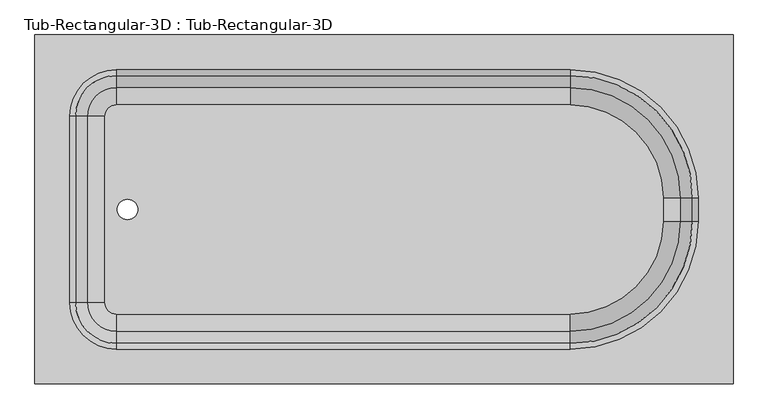
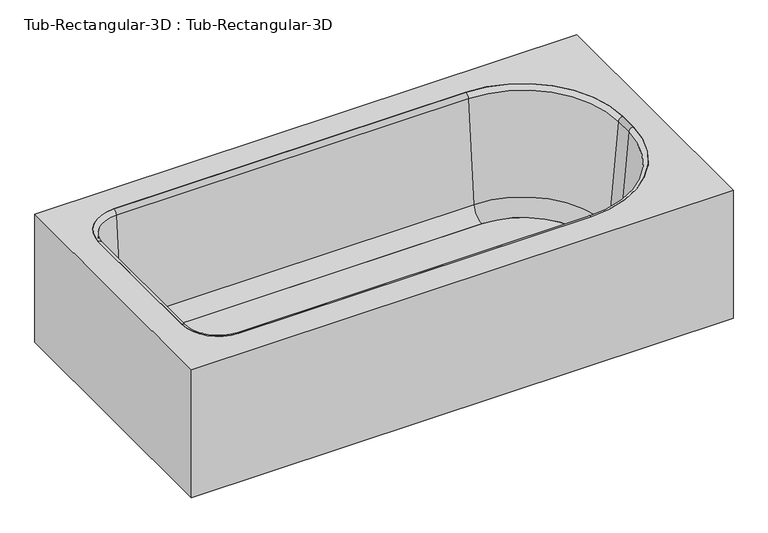
"""IFC4 building model written with IfcOpenShell, lengths in millimetres: flow terminal geometry, Tub-Rectangular-3D : Tub-Rectangular-3D."""

from ifc_helpers import new_model, si_unit, point, frame, frame_2d, origin, place, context, project, spatial, polyline, circle_curve, ellipse_curve, trimmed, segment, composite_curve, outline, extrude, source, transform, mapped, element, save
from ifc_brep_helpers import plane_surface, cylinder_surface, revolved_surface, advanced_brep


def tub_rectangular_3d_tub_rectangular_3d_c1fa07c3(model_context):
    return source(origin(), model_context, "Body", "SolidModel", [
        advanced_brep(
        [(413.3970313, -863.6, 381.0), (413.3970313, -101.6, 381.0), (-1110.6029687, -101.6, 381.0), (-1110.6029687, -863.6, 381.0), (-932.8029687, -787.4, 381.0), (-1034.4029687, -685.8, 381.0), (-1034.4029687, -279.4, 381.0), (-932.8029687, -177.8, 381.0), (57.7970313, -177.8, 381.0), (337.1970313, -457.2, 381.0), (337.1970313, -508.0, 381.0), (57.7970313, -787.4, 381.0), (394.3470313, -844.55, 361.95), (-1091.5529687, -844.55, 361.95), (-1091.5529687, -120.65, 361.95), (394.3470313, -120.65, 361.95), (-932.8029687, -787.4, 361.95), (57.7970313, -787.4, 361.95), (337.1970313, -508.0, 361.95), (337.1970313, -457.2, 361.95), (57.7970313, -177.8, 361.95), (-932.8029687, -177.8, 361.95), (-1034.4029687, -279.4, 361.95), (-1034.4029687, -685.8, 361.95), (-1110.6029687, -863.6, 0.0), (413.3970313, -863.6, 0.0), (-1110.6029687, -101.6, 0.0), (413.3970313, -101.6, 0.0), (394.3470313, -844.55, 0.0), (394.3470313, -120.65, 0.0), (-1091.5529687, -120.65, 0.0), (-1091.5529687, -844.55, 0.0)],
        [
            (0, 1),
            (1, 2),
            (2, 3),
            (3, 0),
            (4, 5, circle_curve(frame((-932.8029687, -685.8, 381.0), z_axis=(0.0, 0.0, -1.0), x_axis=(0.0, -1.0, 0.0)), 101.6)),
            (5, 6),
            (6, 7, circle_curve(frame((-932.8029687, -279.4, 381.0), z_axis=(0.0, 0.0, -1.0), x_axis=(0.0, -1.0, 0.0)), 101.6)),
            (7, 8),
            (8, 9, circle_curve(frame((57.7970313, -457.2, 381.0), z_axis=(0.0, 0.0, -1.0), x_axis=(0.0, -1.0, 0.0)), 279.4)),
            (9, 10),
            (10, 11, circle_curve(frame((57.7970313, -508.0, 381.0), z_axis=(0.0, 0.0, -1.0), x_axis=(0.0, -1.0, 0.0)), 279.4)),
            (11, 4),
            (12, 13),
            (13, 14),
            (14, 15),
            (15, 12),
            (16, 17),
            (17, 18, circle_curve(frame((57.7970313, -508.0, 361.95), z_axis=(0.0, 0.0, 1.0), x_axis=(0.0, -1.0, 0.0)), 279.4)),
            (18, 19),
            (19, 20, circle_curve(frame((57.7970313, -457.2, 361.95), z_axis=(0.0, 0.0, 1.0), x_axis=(0.0, -1.0, 0.0)), 279.4)),
            (20, 21),
            (21, 22, circle_curve(frame((-932.8029687, -279.4, 361.95), z_axis=(0.0, 0.0, 1.0), x_axis=(0.0, -1.0, 0.0)), 101.6)),
            (22, 23),
            (23, 16, circle_curve(frame((-932.8029687, -685.8, 361.95), z_axis=(0.0, 0.0, 1.0), x_axis=(0.0, -1.0, 0.0)), 101.6)),
            (3, 24),
            (24, 25),
            (25, 0),
            (2, 26),
            (26, 24),
            (1, 27),
            (27, 26),
            (25, 27),
            (11, 17),
            (16, 4),
            (10, 18),
            (9, 19),
            (8, 20),
            (7, 21),
            (6, 22),
            (5, 23),
            (28, 29),
            (29, 30),
            (30, 31),
            (31, 28),
            (28, 12),
            (15, 29),
            (14, 30),
            (13, 31),
        ],
        [
            plane_surface(frame((-1110.6029687, -863.6, 381.0), z_axis=(0.0, 0.0, 1.0), x_axis=(-1.0, 0.0, 0.0))),
            plane_surface(frame((-1110.6029687, -863.6, 361.95), z_axis=(0.0, 0.0, -1.0), x_axis=(1.0, 0.0, 0.0))),
            plane_surface(frame((413.3970313, -863.6, 381.0), z_axis=(0.0, -1.0, 0.0), x_axis=(0.0, 0.0, -1.0))),
            plane_surface(frame((-1110.6029687, -863.6, 381.0), z_axis=(-1.0, 0.0, 0.0), x_axis=(0.0, 0.0, -1.0))),
            plane_surface(frame((-1110.6029687, -101.6, 381.0), z_axis=(0.0, 1.0, 0.0), x_axis=(0.0, 0.0, -1.0))),
            plane_surface(frame((413.3970313, -101.6, 381.0), z_axis=(1.0, 0.0, 0.0), x_axis=(0.0, 0.0, -1.0))),
            plane_surface(frame((-932.8029687, -787.4, 381.0), z_axis=(0.0, 1.0, 0.0), x_axis=(0.0, 0.0, -1.0))),
            revolved_surface(polyline([(57.7970313, -787.4, 361.95), (57.7970313, -787.4, 381.0)]), (57.7970313, -508.0, 381.0), (0.0, 0.0, -1.0)),
            plane_surface(frame((337.1970313, -508.0, 381.0), z_axis=(-1.0, 0.0, 0.0), x_axis=(0.0, 0.0, -1.0))),
            revolved_surface(polyline([(57.7970313, -736.5999999999999, 361.95), (57.7970313, -736.5999999999999, 381.0)]), (57.7970313, -457.2, 381.0), (0.0, 0.0, -1.0)),
            plane_surface(frame((57.7970313, -177.8, 381.0), z_axis=(0.0, -1.0, 0.0), x_axis=(0.0, 0.0, -1.0))),
            revolved_surface(polyline([(-932.8029687, -381.0, 361.95), (-932.8029687, -381.0, 381.0)]), (-932.8029687, -279.4, 381.0), (0.0, 0.0, -1.0)),
            plane_surface(frame((-1034.4029687, -279.4, 381.0), z_axis=(1.0, 0.0, 0.0), x_axis=(0.0, 0.0, -1.0))),
            revolved_surface(polyline([(-932.8029687, -787.4, 361.95), (-932.8029687, -787.4, 381.0)]), (-932.8029687, -685.8, 381.0), (0.0, 0.0, -1.0)),
            plane_surface(frame((-1110.6029687, -863.6, 0.0), z_axis=(0.0, 0.0, -1.0), x_axis=(1.0, 0.0, 0.0))),
            plane_surface(frame((394.3470313, -844.55, 361.95), z_axis=(-1.0, 0.0, 0.0), x_axis=(0.0, 0.0, -1.0))),
            plane_surface(frame((394.3470313, -120.65, 361.95), z_axis=(0.0, -1.0, 0.0), x_axis=(0.0, 0.0, -1.0))),
            plane_surface(frame((-1091.5529687, -120.65, 361.95), z_axis=(1.0, 0.0, 0.0), x_axis=(0.0, 0.0, -1.0))),
            plane_surface(frame((-1091.5529687, -844.55, 361.95), z_axis=(0.0, 1.0, 0.0), x_axis=(0.0, 0.0, -1.0))),
        ],
        [
            (0, [[1, 2, 3, 4], [5, 6, 7, 8, 9, 10, 11, 12]]),
            (1, [[13, 14, 15, 16], [17, 18, 19, 20, 21, 22, 23, 24]]),
            (2, [[25, 26, 27, -4]]),
            (3, [[28, 29, -25, -3]]),
            (4, [[30, 31, -28, -2]]),
            (5, [[32, -30, -1, -27]]),
            (6, [[33, -17, 34, -12]]),
            (7, [[35, -18, -33, -11]]),
            (8, [[36, -19, -35, -10]]),
            (9, [[37, -20, -36, -9]]),
            (10, [[38, -21, -37, -8]]),
            (11, [[39, -22, -38, -7]]),
            (12, [[40, -23, -39, -6]]),
            (13, [[-34, -24, -40, -5]]),
            (14, [[-26, -29, -31, -32], [41, 42, 43, 44]]),
            (15, [[45, -16, 46, -41]]),
            (16, [[-46, -15, 47, -42]]),
            (17, [[-47, -14, 48, -43]]),
            (18, [[-48, -13, -45, -44]]),
        ],
    ),
        extrude(outline(composite_curve([segment(polyline([(57.7970313, -710.7964741), (-932.8029687, -710.7964741)]), True, "CONTINUOUS"), segment(trimmed(circle_curve(frame_2d((-932.8029687, -685.8)), 24.9964741), [point((-932.8029687, -710.7964741))], [point((-957.7994428, -685.8))], False, "CARTESIAN"), True, "CONTINUOUS"), segment(polyline([(-957.7994428, -685.8), (-957.7994428, -279.4)]), True, "CONTINUOUS"), segment(trimmed(circle_curve(frame_2d((-932.8029687, -279.4)), 24.9964741), [point((-957.7994428, -279.4))], [point((-932.8029687, -254.4035259))], False, "CARTESIAN"), True, "CONTINUOUS"), segment(polyline([(-932.8029687, -254.4035259), (57.7970313, -254.4035259)]), True, "CONTINUOUS"), segment(trimmed(circle_curve(frame_2d((57.7970313, -457.2)), 202.7964741), [point((57.7970313, -254.4035259))], [point((260.5935054, -457.2))], False, "CARTESIAN"), True, "CONTINUOUS"), segment(polyline([(260.5935054, -457.2), (260.5935054, -508.0)]), True, "CONTINUOUS"), segment(trimmed(circle_curve(frame_2d((57.7970313, -508.0)), 202.7964741), [point((260.5935054, -508.0))], [point((57.7970313, -710.7964741))], False, "CARTESIAN"), True, "CONTINUOUS")], self_intersect=False), holes=[composite_curve([segment(trimmed(circle_curve(frame_2d((-908.510206, -482.6)), 22.225), [point((-908.510206, -504.825))], [point((-908.510206, -460.375))], True, "CARTESIAN"), True, "CONTINUOUS"), segment(trimmed(circle_curve(frame_2d((-908.510206, -482.6)), 22.225), [point((-908.510206, -460.375))], [point((-908.510206, -504.825))], True, "CARTESIAN"), True, "CONTINUOUS")], self_intersect=False)]), frame((0.0, 0.0, 16.863573), z_axis=(0.0, 0.0, 1.0), x_axis=(1.0, 0.0, 0.0)), (0.0, 0.0, 1.0), 19.05),
        advanced_brep(
        [(-995.7544608, -685.8, 70.6929392), (-1021.9249722, -685.8, 369.8232535), (-932.8029687, -774.9220035, 369.8232535), (-932.8029687, -748.7514921, 70.6929392), (-957.7994428, -685.8, 35.913573), (-932.8029687, -710.7964741, 35.913573), (-957.7994428, -685.8, 16.863573), (-932.8029687, -710.7964741, 16.863573), (-1034.4029687, -685.8, 16.863573), (-932.8029687, -787.4, 16.863573), (-1034.4029687, -685.8, 381.0), (-932.8029687, -787.4, 381.0), (-995.7544608, -279.4, 70.6929392), (-1021.9249722, -279.4, 369.8232535), (-957.7994428, -279.4, 35.913573), (-957.7994428, -279.4, 16.863573), (-1034.4029687, -279.4, 16.863573), (-1034.4029687, -279.4, 381.0), (-932.8029687, -216.4485079, 70.6929392), (-932.8029687, -190.2779965, 369.8232535), (-932.8029687, -254.4035259, 35.913573), (-932.8029687, -254.4035259, 16.863573), (-932.8029687, -177.8, 16.863573), (-932.8029687, -177.8, 381.0), (57.7970313, -216.4485079, 70.6929392), (57.7970313, -190.2779965, 369.8232535), (57.7970313, -254.4035259, 35.913573), (57.7970313, -254.4035259, 16.863573), (57.7970313, -177.8, 16.863573), (57.7970313, -177.8, 381.0), (298.5485234, -457.2, 70.6929392), (324.7190348, -457.2, 369.8232535), (260.5935054, -457.2, 35.913573), (260.5935054, -457.2, 16.863573), (337.1970313, -457.2, 16.863573), (337.1970313, -457.2, 381.0), (298.5485234, -508.0, 70.6929392), (324.7190348, -508.0, 369.8232535), (260.5935054, -508.0, 35.913573), (260.5935054, -508.0, 16.863573), (337.1970313, -508.0, 16.863573), (337.1970313, -508.0, 381.0), (57.7970313, -748.7514921, 70.6929392), (57.7970313, -774.9220035, 369.8232535), (57.7970313, -710.7964741, 35.913573), (57.7970313, -710.7964741, 16.863573), (57.7970313, -787.4, 16.863573), (57.7970313, -787.4, 381.0)],
        [
            (0, 1),
            (1, 2, circle_curve(frame((-932.8029687, -685.8, 369.8232535), z_axis=(0.0, 0.0, 1.0), x_axis=(0.0, -1.0, 0.0)), 89.1220035)),
            (2, 3),
            (3, 0, circle_curve(frame((-932.8029687, -685.8, 70.6929392), z_axis=(0.0, 0.0, -1.0), x_axis=(0.0, -1.0, 0.0)), 62.9514921)),
            (4, 0, circle_curve(frame((-957.7994428, -685.8, 74.013573), z_axis=(0.0, 1.0, 0.0), x_axis=(1.0, 0.0, 0.0)), 38.1)),
            (3, 5, circle_curve(frame((-932.8029687, -710.7964741, 74.013573), z_axis=(1.0, 0.0, 0.0), x_axis=(0.0, 1.0, 0.0)), 38.1)),
            (5, 4, circle_curve(frame((-932.8029687, -685.8, 35.913573), z_axis=(0.0, 0.0, -1.0), x_axis=(0.0, -1.0, 0.0)), 24.9964741)),
            (6, 4),
            (5, 7),
            (7, 6, circle_curve(frame((-932.8029687, -685.8, 16.863573), z_axis=(0.0, 0.0, -1.0), x_axis=(0.0, -1.0, 0.0)), 24.9964741)),
            (8, 6),
            (7, 9),
            (9, 8, circle_curve(frame((-932.8029687, -685.8, 16.863573), z_axis=(0.0, 0.0, -1.0), x_axis=(0.0, -1.0, 0.0)), 101.6)),
            (10, 8),
            (9, 11),
            (11, 10, circle_curve(frame((-932.8029687, -685.8, 381.0), z_axis=(0.0, 0.0, -1.0), x_axis=(0.0, -1.0, 0.0)), 101.6)),
            (1, 10, circle_curve(frame((-1034.4029687, -685.8, 368.4462547), z_axis=(0.0, -1.0, 0.0), x_axis=(1.0, 0.0, 0.0)), 12.5537453)),
            (11, 2, circle_curve(frame((-932.8029687, -787.4, 368.4462547), z_axis=(-1.0, 0.0, 0.0), x_axis=(0.0, 1.0, 0.0)), 12.5537453)),
            (0, 12),
            (12, 13),
            (13, 1),
            (4, 14),
            (14, 12, circle_curve(frame((-957.7994428, -279.4, 74.013573), z_axis=(0.0, 1.0, 0.0), x_axis=(1.0, 0.0, 0.0)), 38.1)),
            (6, 15),
            (15, 14),
            (8, 16),
            (16, 15),
            (10, 17),
            (17, 16),
            (13, 17, circle_curve(frame((-1034.4029687, -279.4, 368.4462547), z_axis=(0.0, -1.0, 0.0), x_axis=(1.0, 0.0, 0.0)), 12.5537453)),
            (18, 19),
            (19, 13, circle_curve(frame((-932.8029687, -279.4, 369.8232535), z_axis=(0.0, 0.0, 1.0), x_axis=(-1.0, 0.0, 0.0)), 89.1220035)),
            (12, 18, circle_curve(frame((-932.8029687, -279.4, 70.6929392), z_axis=(0.0, 0.0, -1.0), x_axis=(-1.0, 0.0, 0.0)), 62.9514921)),
            (20, 18, circle_curve(frame((-932.8029687, -254.4035259, 74.013573), z_axis=(1.0, 0.0, 0.0), x_axis=(0.0, -1.0, 0.0)), 38.1)),
            (14, 20, circle_curve(frame((-932.8029687, -279.4, 35.913573), z_axis=(0.0, 0.0, -1.0), x_axis=(-1.0, 0.0, 0.0)), 24.9964741)),
            (21, 20),
            (15, 21, circle_curve(frame((-932.8029687, -279.4, 16.863573), z_axis=(0.0, 0.0, -1.0), x_axis=(-1.0, 0.0, 0.0)), 24.9964741)),
            (22, 21),
            (16, 22, circle_curve(frame((-932.8029687, -279.4, 16.863573), z_axis=(0.0, 0.0, -1.0), x_axis=(-1.0, 0.0, 0.0)), 101.6)),
            (23, 22),
            (17, 23, circle_curve(frame((-932.8029687, -279.4, 381.0), z_axis=(0.0, 0.0, -1.0), x_axis=(-1.0, 0.0, 0.0)), 101.6)),
            (19, 23, circle_curve(frame((-932.8029687, -177.8, 368.4462547), z_axis=(-1.0, 0.0, 0.0), x_axis=(0.0, -1.0, 0.0)), 12.5537453)),
            (18, 24),
            (24, 25),
            (25, 19),
            (20, 26),
            (26, 24, circle_curve(frame((57.7970313, -254.4035259, 74.013573), z_axis=(1.0, 0.0, 0.0), x_axis=(0.0, -1.0, 0.0)), 38.1)),
            (21, 27),
            (27, 26),
            (22, 28),
            (28, 27),
            (23, 29),
            (29, 28),
            (25, 29, circle_curve(frame((57.7970313, -177.8, 368.4462547), z_axis=(-1.0, 0.0, 0.0), x_axis=(0.0, -1.0, 0.0)), 12.5537453)),
            (30, 31),
            (31, 25, circle_curve(frame((57.7970313, -457.2, 369.8232535), z_axis=(0.0, 0.0, 1.0), x_axis=(0.0, 1.0, 0.0)), 266.9220035)),
            (24, 30, circle_curve(frame((57.7970313, -457.2, 70.6929392), z_axis=(0.0, 0.0, -1.0), x_axis=(0.0, 1.0, 0.0)), 240.7514921)),
            (32, 30, circle_curve(frame((260.5935054, -457.2, 74.013573), z_axis=(0.0, -1.0, 0.0), x_axis=(-1.0, 0.0, 0.0)), 38.1)),
            (26, 32, circle_curve(frame((57.7970313, -457.2, 35.913573), z_axis=(0.0, 0.0, -1.0), x_axis=(0.0, 1.0, 0.0)), 202.7964741)),
            (33, 32),
            (27, 33, circle_curve(frame((57.7970313, -457.2, 16.863573), z_axis=(0.0, 0.0, -1.0), x_axis=(0.0, 1.0, 0.0)), 202.7964741)),
            (34, 33),
            (28, 34, circle_curve(frame((57.7970313, -457.2, 16.863573), z_axis=(0.0, 0.0, -1.0), x_axis=(0.0, 1.0, 0.0)), 279.4)),
            (35, 34),
            (29, 35, circle_curve(frame((57.7970313, -457.2, 381.0), z_axis=(0.0, 0.0, -1.0), x_axis=(0.0, 1.0, 0.0)), 279.4)),
            (31, 35, circle_curve(frame((337.1970313, -457.2, 368.4462547), z_axis=(0.0, 1.0, 0.0), x_axis=(-1.0, 0.0, 0.0)), 12.5537453)),
            (30, 36),
            (36, 37),
            (37, 31),
            (32, 38),
            (38, 36, circle_curve(frame((260.5935054, -508.0, 74.013573), z_axis=(0.0, -1.0, 0.0), x_axis=(-1.0, 0.0, 0.0)), 38.1)),
            (33, 39),
            (39, 38),
            (34, 40),
            (40, 39),
            (35, 41),
            (41, 40),
            (37, 41, circle_curve(frame((337.1970313, -508.0, 368.4462547), z_axis=(0.0, 1.0, 0.0), x_axis=(-1.0, 0.0, 0.0)), 12.5537453)),
            (42, 43),
            (43, 37, circle_curve(frame((57.7970313, -508.0, 369.8232535), z_axis=(0.0, 0.0, 1.0), x_axis=(1.0, 0.0, 0.0)), 266.9220035)),
            (36, 42, circle_curve(frame((57.7970313, -508.0, 70.6929392), z_axis=(0.0, 0.0, -1.0), x_axis=(1.0, 0.0, 0.0)), 240.7514921)),
            (44, 42, circle_curve(frame((57.7970313, -710.7964741, 74.013573), z_axis=(-1.0, 0.0, 0.0), x_axis=(0.0, 1.0, 0.0)), 38.1)),
            (38, 44, circle_curve(frame((57.7970313, -508.0, 35.913573), z_axis=(0.0, 0.0, -1.0), x_axis=(1.0, 0.0, 0.0)), 202.7964741)),
            (45, 44),
            (39, 45, circle_curve(frame((57.7970313, -508.0, 16.863573), z_axis=(0.0, 0.0, -1.0), x_axis=(1.0, 0.0, 0.0)), 202.7964741)),
            (46, 45),
            (40, 46, circle_curve(frame((57.7970313, -508.0, 16.863573), z_axis=(0.0, 0.0, -1.0), x_axis=(1.0, 0.0, 0.0)), 279.4)),
            (47, 46),
            (41, 47, circle_curve(frame((57.7970313, -508.0, 381.0), z_axis=(0.0, 0.0, -1.0), x_axis=(1.0, 0.0, 0.0)), 279.4)),
            (43, 47, circle_curve(frame((57.7970313, -787.4, 368.4462547), z_axis=(1.0, 0.0, 0.0), x_axis=(0.0, 1.0, 0.0)), 12.5537453)),
            (42, 3),
            (2, 43),
            (44, 5),
            (45, 7),
            (46, 9),
            (47, 11),
        ],
        [
            revolved_surface(polyline([(-932.8029687, -774.9220035, 369.8232535), (-932.8029687, -748.7514921, 70.6929392)]), (-932.8029687, -685.8, 381.0), (0.0, 0.0, 1.0)),
            revolved_surface(trimmed(ellipse_curve(frame((-932.8029687, -710.7964741, 74.013573), z_axis=(1.0, 0.0, 0.0), x_axis=(0.0, 1.0, 0.0)), 38.1, 38.1), [point((-932.8029687, -748.7514921, 70.6929392))], [point((-932.8029687, -710.7964741, 35.913573))], True, "CARTESIAN"), (-932.8029687, -685.8, 381.0), (0.0, 0.0, 1.0)),
            revolved_surface(polyline([(-932.8029687, -710.7964741, 35.913572999999985), (-932.8029687, -710.7964741, 16.863572999999974)]), (-932.8029687, -685.8, 381.0), (0.0, 0.0, 1.0)),
            plane_surface(frame((-932.8029687, -685.8, 16.863573), z_axis=(0.0, 0.0, -1.0), x_axis=(0.0, -1.0, 0.0))),
            cylinder_surface(frame((-932.8029687, -685.8, 381.0), z_axis=(0.0, 0.0, 1.0), x_axis=(0.0, -1.0, 0.0)), 101.6),
            revolved_surface(trimmed(ellipse_curve(frame((-932.8029687, -787.4, 368.4462547), z_axis=(-1.0, 0.0, 0.0), x_axis=(0.0, 1.0, 0.0)), 12.5537453, 12.5537453), [point((-932.8029687, -787.4, 381.0))], [point((-932.8029687, -774.9220035, 369.8232535))], True, "CARTESIAN"), (-932.8029687, -685.8, 381.0), (0.0, 0.0, 1.0)),
            plane_surface(frame((-1021.9249722, -685.8, 369.8232535), z_axis=(0.9961946980917458, 0.0, 0.08715574274765589), x_axis=(0.0, 1.0, 0.0))),
            revolved_surface(polyline([(-919.6994427999999, -279.4, 74.013573), (-919.6994427999999, -685.8, 74.013573)]), (-957.7994428, -685.8, 74.013573), (0.0, 1.0, 0.0)),
            plane_surface(frame((-957.7994428, -685.8, 35.913573), z_axis=(1.0, 0.0, 0.0), x_axis=(0.0, 1.0, 0.0))),
            plane_surface(frame((-957.7994428, -685.8, 16.863573), z_axis=(0.0, 0.0, -1.0), x_axis=(0.0, 1.0, 0.0))),
            plane_surface(frame((-1034.4029687, -685.8, 16.863573), z_axis=(-1.0, 0.0, 0.0), x_axis=(0.0, 1.0, 0.0))),
            cylinder_surface(frame((-1034.4029687, -685.8, 368.4462547), z_axis=(0.0, -1.0, 0.0), x_axis=(1.0, 0.0, 0.0)), 12.5537453),
            revolved_surface(polyline([(-1021.9249722, -279.4, 369.8232535), (-995.7544608, -279.4, 70.6929392)]), (-932.8029687, -279.4, 381.0), (0.0, 0.0, 1.0)),
            revolved_surface(trimmed(ellipse_curve(frame((-957.7994428, -279.4, 74.013573), z_axis=(0.0, -1.0, 0.0), x_axis=(1.0, 0.0, 0.0)), 38.1, 38.1), [point((-995.7544608, -279.4, 70.6929392))], [point((-957.7994428, -279.4, 35.913573))], True, "CARTESIAN"), (-932.8029687, -279.4, 381.0), (0.0, 0.0, 1.0)),
            revolved_surface(polyline([(-957.7994428, -279.4, 35.913572999999985), (-957.7994428, -279.4, 16.863572999999974)]), (-932.8029687, -279.4, 381.0), (0.0, 0.0, 1.0)),
            plane_surface(frame((-932.8029687, -279.4, 16.863573), z_axis=(0.0, 0.0, -1.0), x_axis=(-1.0, 0.0, 0.0))),
            cylinder_surface(frame((-932.8029687, -279.4, 381.0), z_axis=(0.0, 0.0, 1.0), x_axis=(-1.0, 0.0, 0.0)), 101.6),
            revolved_surface(trimmed(ellipse_curve(frame((-1034.4029687, -279.4, 368.4462547), z_axis=(0.0, 1.0, 0.0), x_axis=(1.0, 0.0, 0.0)), 12.5537453, 12.5537453), [point((-1034.4029687, -279.4, 381.0))], [point((-1021.9249722, -279.4, 369.8232535))], True, "CARTESIAN"), (-932.8029687, -279.4, 381.0), (0.0, 0.0, 1.0)),
            plane_surface(frame((-932.8029687, -190.2779965, 369.8232535), z_axis=(0.0, -0.9961946980917461, 0.08715574274765266), x_axis=(1.0, 0.0, 0.0))),
            revolved_surface(polyline([(57.79703129999996, -292.5035259, 74.013573), (-932.8029687, -292.5035259, 74.013573)]), (-932.8029687, -254.4035259, 74.013573), (1.0, 0.0, 0.0)),
            plane_surface(frame((-932.8029687, -254.4035259, 35.913573), z_axis=(0.0, -1.0, 0.0), x_axis=(1.0, 0.0, 0.0))),
            plane_surface(frame((-932.8029687, -254.4035259, 16.863573), z_axis=(0.0, 0.0, -1.0), x_axis=(1.0, 0.0, 0.0))),
            plane_surface(frame((-932.8029687, -177.8, 16.863573), z_axis=(0.0, 1.0, 0.0), x_axis=(1.0, 0.0, 0.0))),
            cylinder_surface(frame((-932.8029687, -177.8, 368.4462547), z_axis=(-1.0, 0.0, 0.0), x_axis=(0.0, -1.0, 0.0)), 12.5537453),
            revolved_surface(polyline([(57.7970313, -190.2779965, 369.8232535), (57.7970313, -216.4485079, 70.6929392)]), (57.7970313, -457.2, 381.0), (0.0, 0.0, 1.0)),
            revolved_surface(trimmed(ellipse_curve(frame((57.7970313, -254.4035259, 74.013573), z_axis=(-1.0, 0.0, 0.0), x_axis=(0.0, -1.0, 0.0)), 38.1, 38.1), [point((57.7970313, -216.4485079, 70.6929392))], [point((57.7970313, -254.4035259, 35.913573))], True, "CARTESIAN"), (57.7970313, -457.2, 381.0), (0.0, 0.0, 1.0)),
            revolved_surface(polyline([(57.7970313, -254.40352589999998, 35.913572999999985), (57.7970313, -254.40352589999998, 16.863572999999974)]), (57.7970313, -457.2, 381.0), (0.0, 0.0, 1.0)),
            plane_surface(frame((57.7970313, -457.2, 16.863573), z_axis=(0.0, 0.0, -1.0), x_axis=(0.0, 1.0, 0.0))),
            cylinder_surface(frame((57.7970313, -457.2, 381.0), z_axis=(0.0, 0.0, 1.0), x_axis=(0.0, 1.0, 0.0)), 279.4),
            revolved_surface(trimmed(ellipse_curve(frame((57.7970313, -177.8, 368.4462547), z_axis=(1.0, 0.0, 0.0), x_axis=(0.0, -1.0, 0.0)), 12.5537453, 12.5537453), [point((57.7970313, -177.8, 381.0))], [point((57.7970313, -190.2779965, 369.8232535))], True, "CARTESIAN"), (57.7970313, -457.2, 381.0), (0.0, 0.0, 1.0)),
            plane_surface(frame((324.7190348, -457.2, 369.8232535), z_axis=(-0.9961946980917464, 0.0, 0.08715574274764942), x_axis=(0.0, -1.0, 0.0))),
            revolved_surface(polyline([(222.49350540000003, -508.0, 74.013573), (222.49350540000003, -457.2, 74.013573)]), (260.5935054, -457.2, 74.013573), (0.0, -1.0, 0.0)),
            plane_surface(frame((260.5935054, -457.2, 35.913573), z_axis=(-1.0, 0.0, 0.0), x_axis=(0.0, -1.0, 0.0))),
            plane_surface(frame((260.5935054, -457.2, 16.863573), z_axis=(0.0, 0.0, -1.0), x_axis=(0.0, -1.0, 0.0))),
            plane_surface(frame((337.1970313, -457.2, 16.863573), z_axis=(1.0, 0.0, 0.0), x_axis=(0.0, -1.0, 0.0))),
            cylinder_surface(frame((337.1970313, -457.2, 368.4462547), z_axis=(0.0, 1.0, 0.0), x_axis=(-1.0, 0.0, 0.0)), 12.5537453),
            revolved_surface(polyline([(324.7190348, -508.0, 369.8232535), (298.5485234, -508.0, 70.6929392)]), (57.7970313, -508.0, 381.0), (0.0, 0.0, 1.0)),
            revolved_surface(trimmed(ellipse_curve(frame((260.5935054, -508.0, 74.013573), z_axis=(0.0, 1.0, 0.0), x_axis=(-1.0, 0.0, 0.0)), 38.1, 38.1), [point((298.5485234, -508.0, 70.6929392))], [point((260.5935054, -508.0, 35.913573))], True, "CARTESIAN"), (57.7970313, -508.0, 381.0), (0.0, 0.0, 1.0)),
            revolved_surface(polyline([(260.5935054, -508.0, 35.913572999999985), (260.5935054, -508.0, 16.863572999999974)]), (57.7970313, -508.0, 381.0), (0.0, 0.0, 1.0)),
            plane_surface(frame((57.7970313, -508.0, 16.863573), z_axis=(0.0, 0.0, -1.0), x_axis=(1.0, 0.0, 0.0))),
            cylinder_surface(frame((57.7970313, -508.0, 381.0), z_axis=(0.0, 0.0, 1.0), x_axis=(1.0, 0.0, 0.0)), 279.4),
            revolved_surface(trimmed(ellipse_curve(frame((337.1970313, -508.0, 368.4462547), z_axis=(0.0, -1.0, 0.0), x_axis=(-1.0, 0.0, 0.0)), 12.5537453, 12.5537453), [point((337.1970313, -508.0, 381.0))], [point((324.7190348, -508.0, 369.8232535))], True, "CARTESIAN"), (57.7970313, -508.0, 381.0), (0.0, 0.0, 1.0)),
            plane_surface(frame((57.7970313, -774.9220035, 369.8232535), z_axis=(0.0, 0.9961946980917461, 0.08715574274765266), x_axis=(-1.0, 0.0, 0.0))),
            revolved_surface(polyline([(-932.8029687, -672.6964740999999, 74.013573), (57.7970313, -672.6964740999999, 74.013573)]), (57.7970313, -710.7964741, 74.013573), (-1.0, 0.0, 0.0)),
            plane_surface(frame((57.7970313, -710.7964741, 35.913573), z_axis=(0.0, 1.0, 0.0), x_axis=(-1.0, 0.0, 0.0))),
            plane_surface(frame((57.7970313, -710.7964741, 16.863573), z_axis=(0.0, 0.0, -1.0), x_axis=(-1.0, 0.0, 0.0))),
            plane_surface(frame((57.7970313, -787.4, 16.863573), z_axis=(0.0, -1.0, 0.0), x_axis=(-1.0, 0.0, 0.0))),
            cylinder_surface(frame((57.7970313, -787.4, 368.4462547), z_axis=(1.0, 0.0, 0.0), x_axis=(0.0, 1.0, 0.0)), 12.5537453),
        ],
        [
            (0, [[1, 2, 3, 4]]),
            (1, [[5, -4, 6, 7]]),
            (2, [[8, -7, 9, 10]]),
            (3, [[11, -10, 12, 13]]),
            (4, [[14, -13, 15, 16]]),
            (5, [[17, -16, 18, -2]]),
            (6, [[19, 20, 21, -1]]),
            (7, [[22, 23, -19, -5]]),
            (8, [[24, 25, -22, -8]]),
            (9, [[26, 27, -24, -11]]),
            (10, [[28, 29, -26, -14]]),
            (11, [[-21, 30, -28, -17]]),
            (12, [[31, 32, -20, 33]]),
            (13, [[34, -33, -23, 35]]),
            (14, [[36, -35, -25, 37]]),
            (15, [[38, -37, -27, 39]]),
            (16, [[40, -39, -29, 41]]),
            (17, [[42, -41, -30, -32]]),
            (18, [[43, 44, 45, -31]]),
            (19, [[46, 47, -43, -34]]),
            (20, [[48, 49, -46, -36]]),
            (21, [[50, 51, -48, -38]]),
            (22, [[52, 53, -50, -40]]),
            (23, [[-45, 54, -52, -42]]),
            (24, [[55, 56, -44, 57]]),
            (25, [[58, -57, -47, 59]]),
            (26, [[60, -59, -49, 61]]),
            (27, [[62, -61, -51, 63]]),
            (28, [[64, -63, -53, 65]]),
            (29, [[66, -65, -54, -56]]),
            (30, [[67, 68, 69, -55]]),
            (31, [[70, 71, -67, -58]]),
            (32, [[72, 73, -70, -60]]),
            (33, [[74, 75, -72, -62]]),
            (34, [[76, 77, -74, -64]]),
            (35, [[-69, 78, -76, -66]]),
            (36, [[79, 80, -68, 81]]),
            (37, [[82, -81, -71, 83]]),
            (38, [[84, -83, -73, 85]]),
            (39, [[86, -85, -75, 87]]),
            (40, [[88, -87, -77, 89]]),
            (41, [[90, -89, -78, -80]]),
            (42, [[91, -3, 92, -79]]),
            (43, [[93, -6, -91, -82]]),
            (44, [[94, -9, -93, -84]]),
            (45, [[95, -12, -94, -86]]),
            (46, [[96, -15, -95, -88]]),
            (47, [[-92, -18, -96, -90]]),
        ],
    ),
    ])


if __name__ == "__main__":
    model = new_model("IFC4")
    model_context = context("Model", 3, world=origin())
    ifc_project = project(units=[si_unit("LENGTHUNIT", "METRE", prefix="MILLI")], contexts=[model_context])
    site = spatial("IfcSite", under=ifc_project)
    building = spatial("IfcBuilding", under=site)
    placement = place(None, origin())
    tub_rectangular_3d_tub_rectangular_3d_shape = tub_rectangular_3d_tub_rectangular_3d_c1fa07c3(model_context)
    element("IfcFlowTerminal", 1, ObjectType="Tub-Rectangular-3D : Tub-Rectangular-3D", at=placement, inside=building, context=model_context, shape_type="MappedRepresentation", body=[
        mapped(tub_rectangular_3d_tub_rectangular_3d_shape, transform((0.0, 0.0, 0.0), x_axis=(1.0, 0.0, 0.0), y_axis=(0.0, 1.0, 0.0), z_axis=(0.0, 0.0, 1.0))),
    ])
    save(model, "model.ifc")

# Revit data of these elements
# Type "Tub-Rectangular-3D : Tub-Rectangular-3D"
#   Assembly Code = "D2010500"
#   Depth = 2' - 6"
#   Height = 1' - 3"
#   Width = 5' - 0"
#   Tub Material = Porcelain, Ivory
#   Default Elevation = 0
# Element 1 (IfcFlowTerminal, "Tub-Rectangular-3D : Tub-Rectangular-3D")
#   Materials on its faces: "Porcelain, Ivory"
# Materials
#   "Porcelain, Ivory": class "Ceramic", colour RGB 247 247 239, transparency 0, Description = "Porcelain, ivory", Cost = 0
